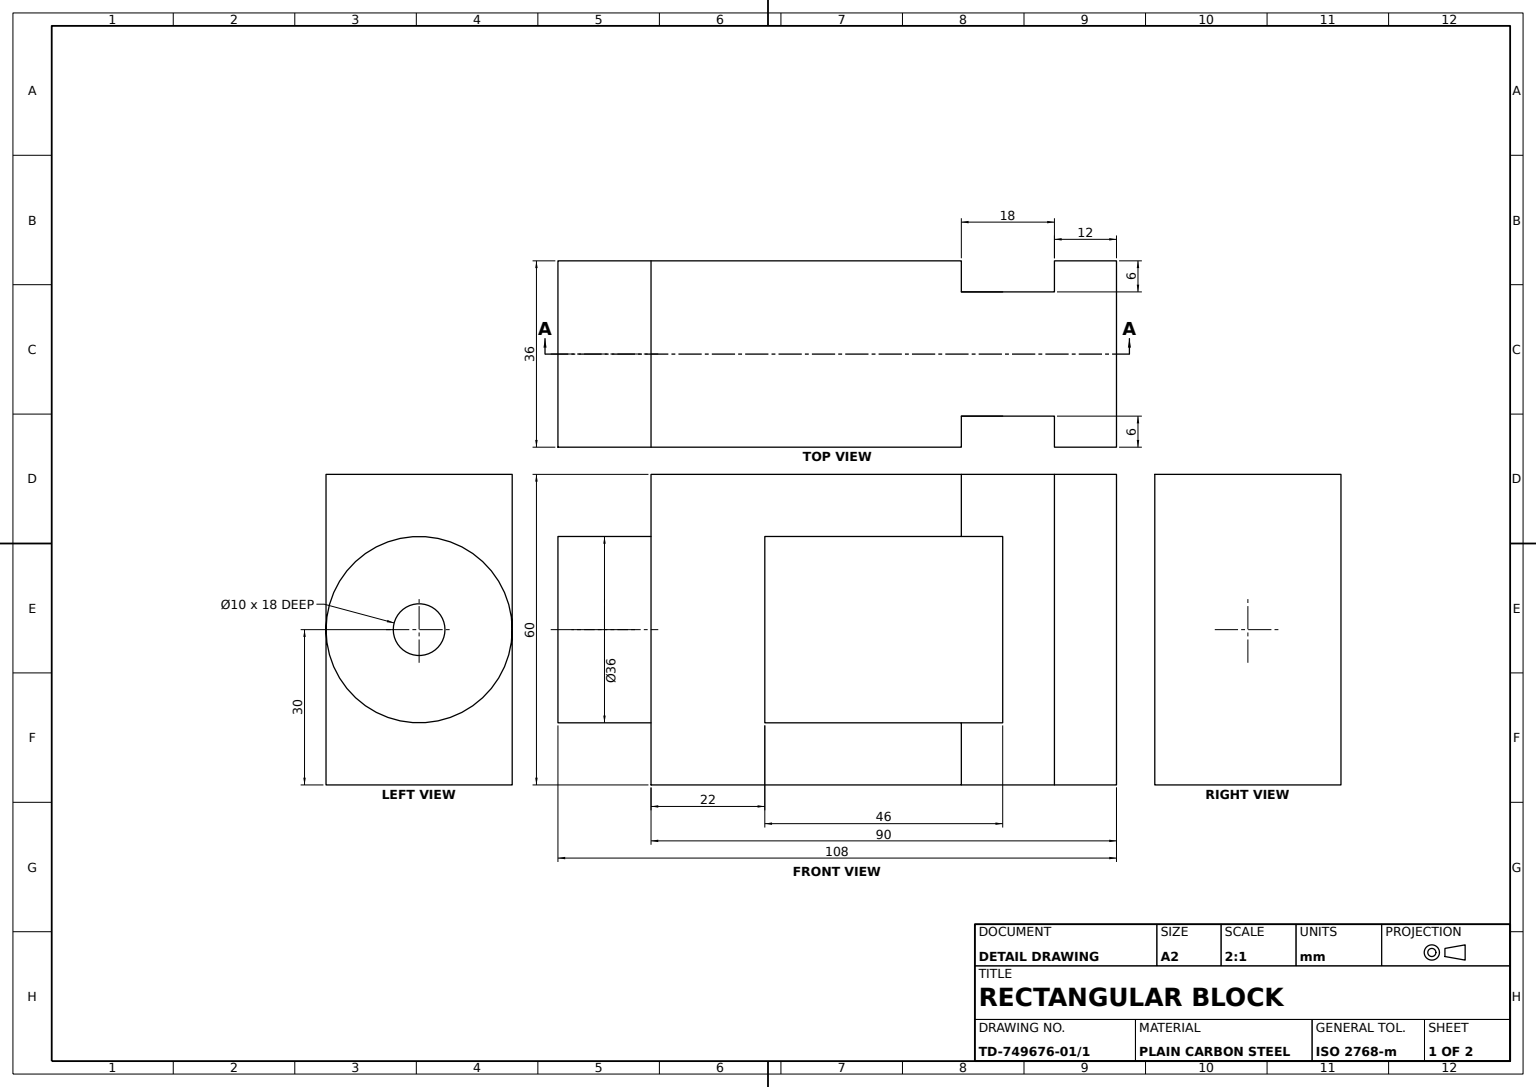
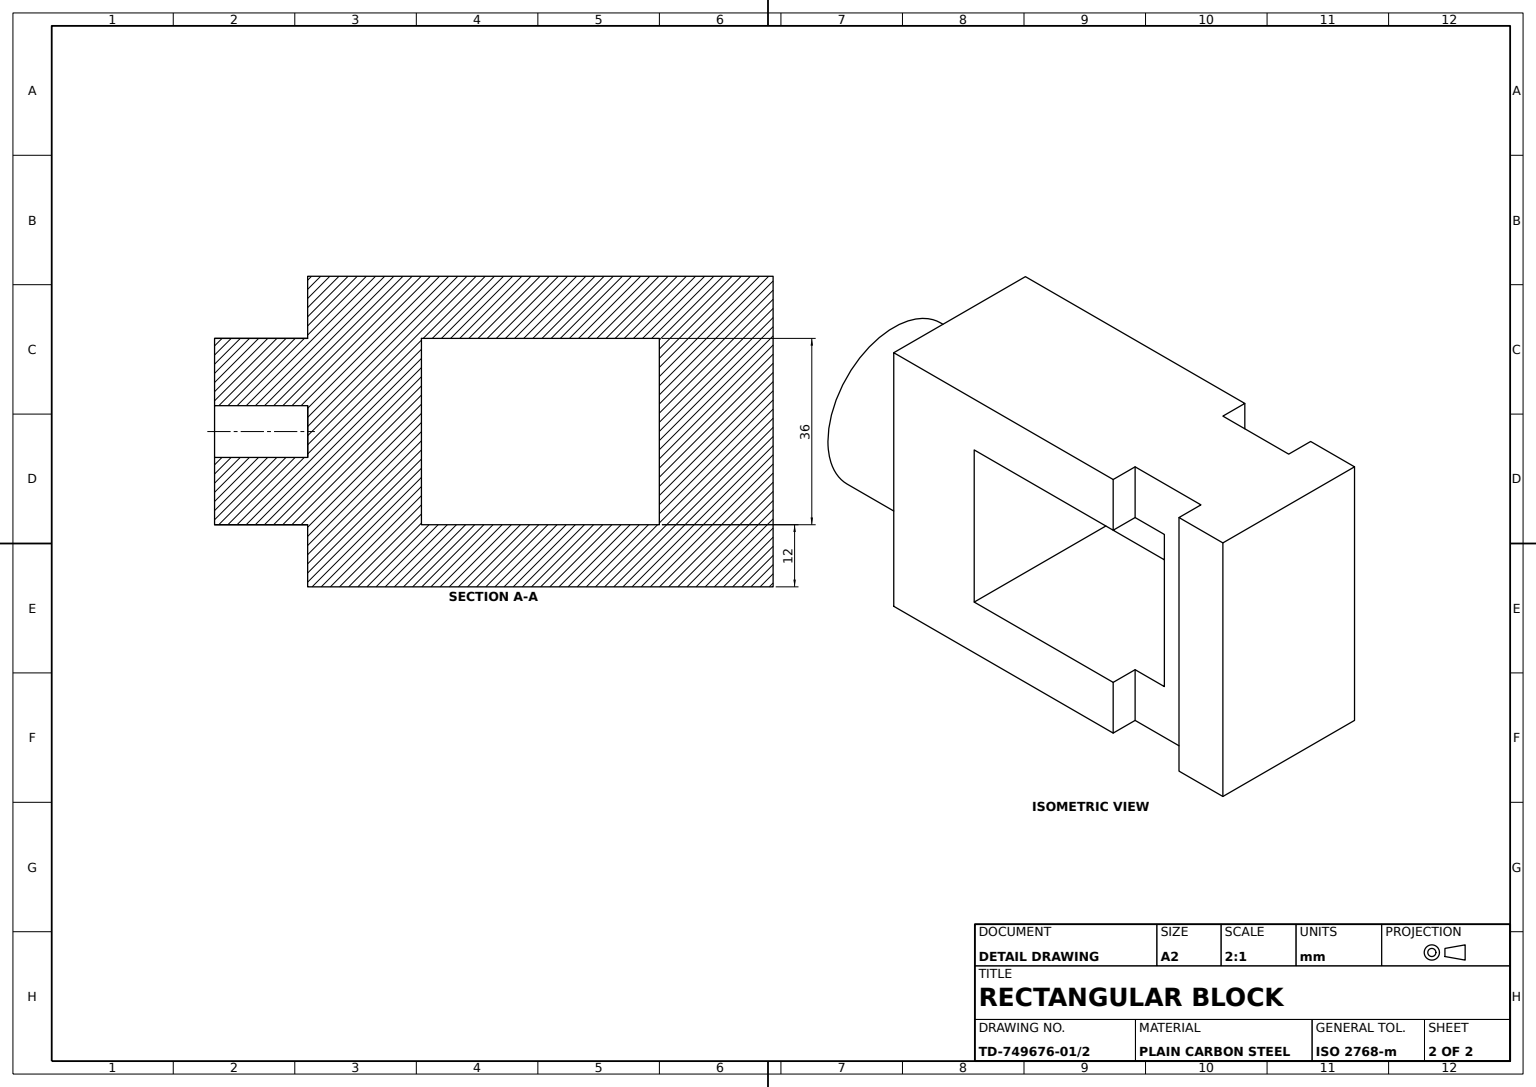
SolidWorks part; units mm, degrees
material "Plain Carbon Steel"
ref_plane "Front Plane" through (0, 0, 0) normal (0, 0, 1) x (1, 0, 0)
ref_plane "Top Plane" through (0, 0, 0) normal (0, 1, 0) x (1, 0, 0)
ref_plane "Right Plane" through (0, 0, 0) normal (1, 0, 0) x (0, 0, -1)
sketch "Base Block Sketch" plane through (0, 0, 0) normal (0, 0, 1) x (1, 0, 0)
  line L0 (-104.5133, 0) -> (106.4602, 0) construction
  line L1 (0, 61.3274) -> (0, -65.7522) construction
  line L3 (-45, -30) -> (45, -30)
  line L4 (-45, -30) -> (-45, 30)
  line L5 (-45, 30) -> (45, 30)
  line L6 (45, -30) -> (45, 30)
  line L7 (-45, -30) -> (45, 30) construction
  line L8 (-45, 30) -> (45, -30) construction
  point P5 (0, 0)
  dimension "D1" = 60
  dimension "D2" = 90
extrude "Base Block" add sketch "Base Block Sketch" along normal blind 36
sketch "Window Sketch" plane through (0, 0, 36) normal (0, 0, 1) x (1, 0, 0)
  line L1 (-23, -18) -> (23, -18)
  line L2 (-23, -18) -> (-23, 18)
  line L3 (-23, 18) -> (23, 18)
  line L4 (23, -18) -> (23, 18)
  line L5 (-23, -18) -> (23, 18) construction
  line L6 (-23, 18) -> (23, -18) construction
  point P0 (0, 0)
  dimension "D1" = 46
  dimension "D2" = 36
extrude "Through Window 46x36" cut sketch "Window Sketch" against normal blind 36
sketch "Boss Sketch" plane through (-45, 0, 0) normal (-1, 0, 0) x (0, 0, 1)
  line L0 (0, 0) -> (36, 0) construction
  line L1 (36, 30) -> (36, -30) construction
  circle A0 centre (18, 0) radius 18
extrude "Cylindrical Boss" add sketch "Boss Sketch" along normal blind 18
sketch "Boss Bore Sketch" plane through (-63, 0, 0) normal (-1, 0, 0) x (0, 0, 1)
  circle A0 centre (18, 0) radius 5
  dimension "D1" = 10
extrude "Boss Bore" cut sketch "Boss Bore Sketch" against normal blind 18
sketch "Top Notches Sketch" plane through (0, -30, 0) normal (0, -1, 0) x (1, 0, 0)
  line L0 (-71.1072, 18) -> (62.2076, 18) construction
  line L1 (45, 36) -> (45, 0) construction
  line L2 (15, 36) -> (33, 36)
  line L3 (15, 36) -> (15, 30)
  line L4 (15, 30) -> (33, 30)
  line L5 (-45, 0) -> (45, 0)
  line L6 (45, 0) -> (45, 36)
  line L7 (45, 36) -> (-45, 36)
  line L8 (-45, 36) -> (-45, 0)
  line L9 (15, 0) -> (33, 0)
  line L11 (33, 36) -> (-45, 36)
  line L13 (33, 36) -> (33, 30)
  line L14 (15, 0) -> (33, 0)
  line L15 (15, 0) -> (15, 6)
  line L16 (15, 6) -> (33, 6)
  line L17 (33, 0) -> (33, 6)
  line M11 (-45, 0) -> (45, 0)
  dimension "D2" = 12
  dimension "D3" = 6
  dimension "D4" = 18
  dimension "D5" = 12
  dimension "D6" = 6
  dimension "D7" = 18
  dimension "D8" = 18
  dimension "D1" = 0
extrude "Top Notches" cut sketch "Top Notches Sketch" against normal through all contours L17 L16 L15 M11
sketch "End Notch Sketch" plane through (0, -30, 0) normal (0, -1, 0) x (1, 0, 0)
  line L0 (-45, 36) -> (45, 36) construction
  line L1 (15, 36) -> (33, 36)
  line L2 (15, 36) -> (15, 30)
  line L3 (15, 30) -> (33, 30)
  line L4 (33, 36) -> (33, 30)
  line L5 (45, 36) -> (45, 0) construction
  dimension "D1" = 12
  dimension "D2" = 18
  dimension "D3" = 6
extrude "End Notch" cut sketch "End Notch Sketch" against normal through all
